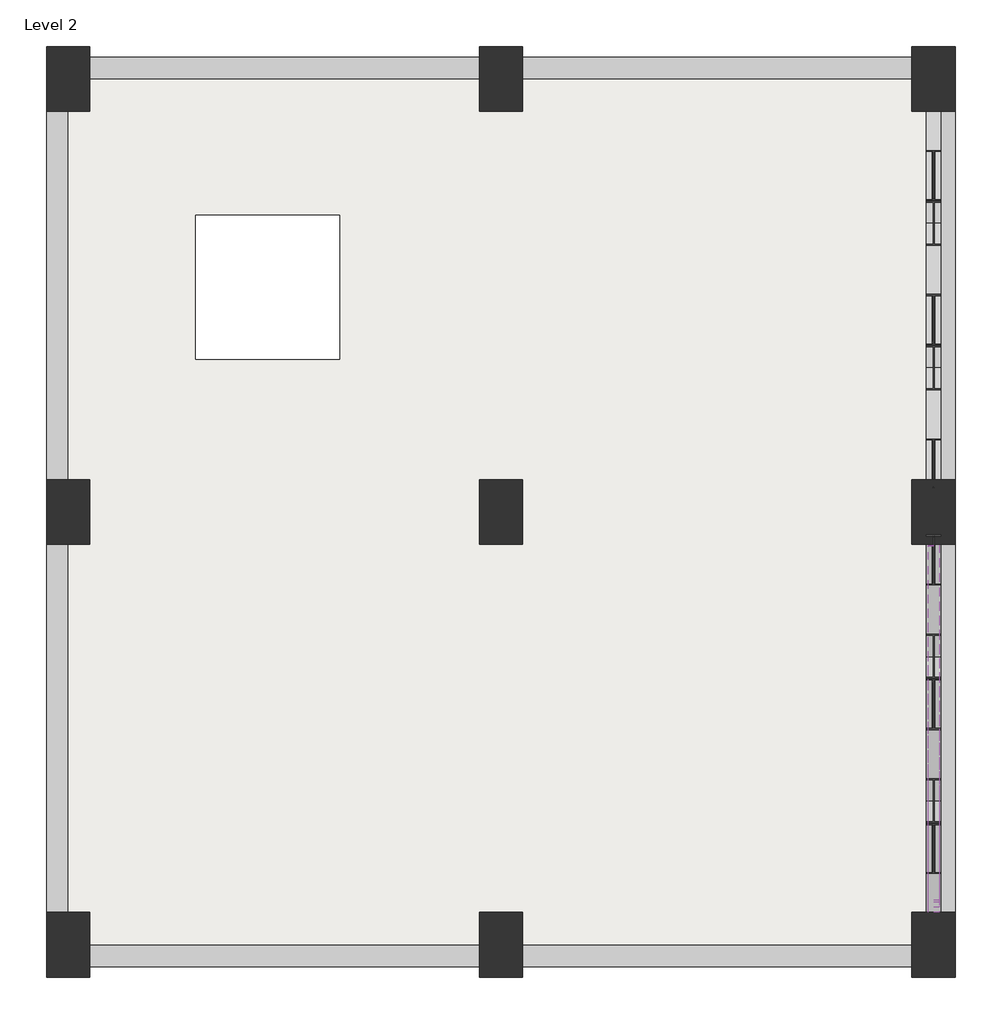
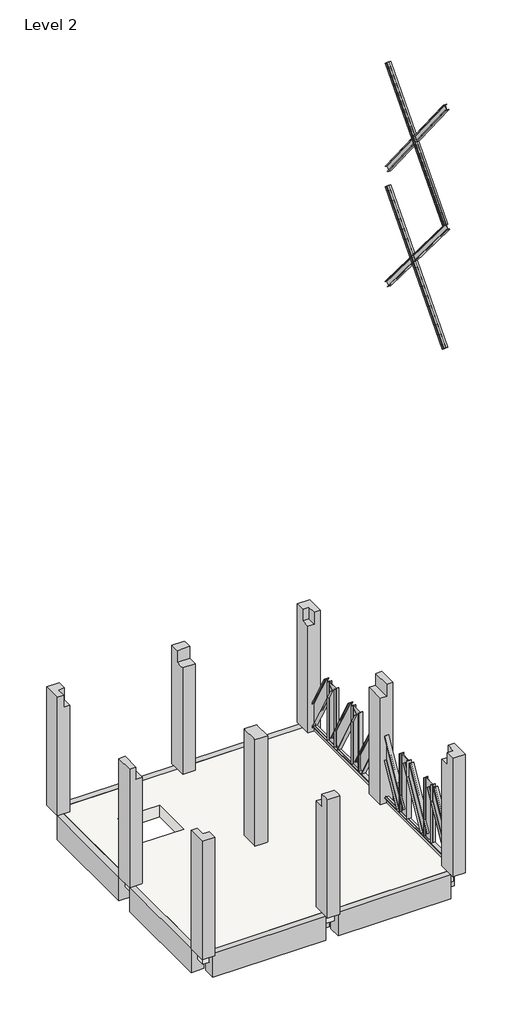
# One storey: 20 beams, 9 columns, 4 members, 1 slab.
"""IFC4 building model written with IfcOpenShell, lengths in millimetres."""

from ifc_helpers import new_model, si_unit, frame, origin, place, context, project, spatial, polyline, outline, extrude, faceted_brep, transform, mapped, element, save
from components import ub_universal_beams_ub305x102x25_07ba02ff, ub_universal_beams_ub305x102x25_e3bd1737, ub_universal_beams_ub305x102x25_1ef2d586, ub_universal_beams_ub305x102x25_1ce1eee3, ub_universal_beams_ub305x102x25_b0bcaaf9, ub_universal_beams_ub305x102x25_8854acc3, ub_universal_beams_ub127x76x13_debcaab1, ub_universal_beams_ub127x76x13_6b492b77, ub_universal_beams_ub127x76x13_5289bed7, ub_universal_beams_ub127x76x13_b97c8348

model = new_model("IFC4")

# Units and contexts
model_context = context("Model", 3, world=origin())
ifc_project = project(units=[si_unit("LENGTHUNIT", "METRE", prefix="MILLI")], contexts=[model_context])

# Site, building, storey
site = spatial("IfcSite", under=ifc_project)
building = spatial("IfcBuilding", under=site)
storey = spatial("IfcBuildingStorey", under=building, Name="Level 2", Elevation=3000.0)

# Beams
placement = place(None, origin())
element("IfcBeam", 1, ObjectType="Concrete-Rectangular Beam : 300 x 600mm", at=placement, inside=storey, context=model_context, shape_type="SweptSolid", body=[
    extrude(outline(polyline([(526.3372902, 2400.0), (226.3372902, 2400.0), (226.3372902, 2700.0), (376.3372902, 2700.0), (376.3372902, 3000.0), (526.3372902, 3000.0), (526.3372902, 2400.0)])), frame((2068.7595868, 0.0, 0.0), z_axis=(1.0, 0.0, 0.0), x_axis=(0.0, 1.0, 0.0)), (0.0, 0.0, 1.0), 2700.0),
    extrude(outline(polyline([(526.3372902, 2400.0), (226.3372902, 2400.0), (226.3372902, 2700.0), (376.3372902, 2700.0), (376.3372902, 3000.0), (526.3372902, 3000.0), (526.3372902, 2400.0)])), frame((-931.2404132, 0.0, 0.0), z_axis=(1.0, 0.0, 0.0), x_axis=(0.0, 1.0, 0.0)), (0.0, 0.0, 1.0), 2700.0),
])
element("IfcBeam", 2, ObjectType="Concrete-Rectangular Beam : 300 x 600mm", at=placement, inside=storey, context=model_context, shape_type="SweptSolid", body=[
    extrude(outline(polyline([(2400.0, 5068.7595868), (3000.0, 5068.7595868), (3000.0, 4918.7595868), (2700.0, 4918.7595868), (2700.0, 4768.7595868), (2400.0, 4768.7595868), (2400.0, 5068.7595868)])), frame((0.0, -2398.6627098, 0.0), z_axis=(0.0, 1.0, 0.0), x_axis=(0.0, 0.0, 1.0)), (0.0, 0.0, 1.0), 2550.0),
    extrude(outline(polyline([(2400.0, 5068.7595868), (3000.0, 5068.7595868), (3000.0, 4918.7595868), (2700.0, 4918.7595868), (2700.0, 4768.7595868), (2400.0, 4768.7595868), (2400.0, 5068.7595868)])), frame((0.0, -5398.6627098, 0.0), z_axis=(0.0, 1.0, 0.0), x_axis=(0.0, 0.0, 1.0)), (0.0, 0.0, 1.0), 2550.0),
])
element("IfcBeam", 3, ObjectType="Concrete-Rectangular Beam : 300 x 600mm", at=placement, inside=storey, context=model_context, shape_type="SweptSolid", body=[
    extrude(outline(polyline([(-5773.6627098, 2400.0), (-5773.6627098, 3000.0), (-5623.6627098, 3000.0), (-5623.6627098, 2700.0), (-5473.6627098, 2700.0), (-5473.6627098, 2400.0), (-5773.6627098, 2400.0)])), frame((2068.7595868, 0.0, 0.0), z_axis=(1.0, 0.0, 0.0), x_axis=(0.0, 1.0, 0.0)), (0.0, 0.0, 1.0), 2700.0),
    extrude(outline(polyline([(-5773.6627098, 2400.0), (-5773.6627098, 3000.0), (-5623.6627098, 3000.0), (-5623.6627098, 2700.0), (-5473.6627098, 2700.0), (-5473.6627098, 2400.0), (-5773.6627098, 2400.0)])), frame((-931.2404132, 0.0, 0.0), z_axis=(1.0, 0.0, 0.0), x_axis=(0.0, 1.0, 0.0)), (0.0, 0.0, 1.0), 2700.0),
])
element("IfcBeam", 4, ObjectType="Concrete-Rectangular Beam : 300 x 600mm", at=placement, inside=storey, context=model_context, shape_type="SweptSolid", body=[
    extrude(outline(polyline([(3000.0, -1231.2404132), (2400.0, -1231.2404132), (2400.0, -931.2404132), (2700.0, -931.2404132), (2700.0, -1081.2404132), (3000.0, -1081.2404132), (3000.0, -1231.2404132)])), frame((0.0, -5398.6627098, 0.0), z_axis=(0.0, 1.0, 0.0), x_axis=(0.0, 0.0, 1.0)), (0.0, 0.0, 1.0), 2550.0),
    extrude(outline(polyline([(3000.0, -1231.2404132), (2400.0, -1231.2404132), (2400.0, -931.2404132), (2700.0, -931.2404132), (2700.0, -1081.2404132), (3000.0, -1081.2404132), (3000.0, -1231.2404132)])), frame((0.0, -2398.6627098, 0.0), z_axis=(0.0, 1.0, 0.0), x_axis=(0.0, 0.0, 1.0)), (0.0, 0.0, 1.0), 2550.0),
])
element("IfcBeam", 5, ObjectType="Concrete-Rectangular Beam : 300 x 600mm", at=placement, inside=storey, context=model_context, shape_type="SweptSolid", body=[
    extrude(outline(polyline([(2068.7595868, -5398.6627098), (1768.7595868, -5398.6627098), (1768.7595868, -2848.6627098), (2068.7595868, -2848.6627098), (2068.7595868, -5398.6627098)])), frame((0.0, 0.0, 2400.0), z_axis=(0.0, 0.0, 1.0), x_axis=(1.0, 0.0, 0.0)), (0.0, 0.0, 1.0), 300.0),
    extrude(outline(polyline([(1768.7595868, 151.3372902), (2068.7595868, 151.3372902), (2068.7595868, -2398.6627098), (1768.7595868, -2398.6627098), (1768.7595868, 151.3372902)])), frame((0.0, 0.0, 2400.0), z_axis=(0.0, 0.0, 1.0), x_axis=(1.0, 0.0, 0.0)), (0.0, 0.0, 1.0), 300.0),
])
element("IfcBeam", 6, ObjectType="Concrete-Rectangular Beam : 300 x 600mm", at=placement, inside=storey, context=model_context, shape_type="SweptSolid", body=[
    extrude(outline(polyline([(4768.7595868, -2473.6627098), (4768.7595868, -2773.6627098), (2068.7595868, -2773.6627098), (2068.7595868, -2473.6627098), (4768.7595868, -2473.6627098)])), frame((0.0, 0.0, 2400.0), z_axis=(0.0, 0.0, 1.0), x_axis=(1.0, 0.0, 0.0)), (0.0, 0.0, 1.0), 300.0),
    extrude(outline(polyline([(-931.2404132, -2773.6627098), (-931.2404132, -2473.6627098), (1768.7595868, -2473.6627098), (1768.7595868, -2773.6627098), (-931.2404132, -2773.6627098)])), frame((0.0, 0.0, 2400.0), z_axis=(0.0, 0.0, 1.0), x_axis=(1.0, 0.0, 0.0)), (0.0, 0.0, 1.0), 300.0),
])
ub_universal_beams_ub305x102x25_shape = ub_universal_beams_ub305x102x25_07ba02ff(model_context)
element("IfcBeam", 7, ObjectType="UB-Universal Beams : UB305x102x25", at=placement, inside=storey, context=model_context, shape_type="MappedRepresentation", body=[
    mapped(ub_universal_beams_ub305x102x25_shape, transform((4918.7595868, -2623.6627098, 3000.0), x_axis=(0.0, 1.0, 0.0), y_axis=(-1.0, 0.0, 0.0), z_axis=(0.0, 0.0, 1.0))),
])
ub_universal_beams_ub305x102x25_2_shape = ub_universal_beams_ub305x102x25_e3bd1737(model_context)
element("IfcBeam", 8, ObjectType="UB-Universal Beams : UB305x102x25", at=placement, inside=storey, context=model_context, shape_type="MappedRepresentation", body=[
    mapped(ub_universal_beams_ub305x102x25_2_shape, transform((4918.7595868, -5623.6627098, 3900.0), x_axis=(0.0, 0.0, 1.0), y_axis=(1.0, 0.0, 0.0), z_axis=(0.0, 1.0, 0.0))),
])
element("IfcBeam", 9, ObjectType="UB-Universal Beams : UB305x102x25", at=placement, inside=storey, context=model_context, shape_type="MappedRepresentation", body=[
    mapped(ub_universal_beams_ub305x102x25_2_shape, transform((4918.7595868, -2623.6627098, 3900.0), x_axis=(0.0, 0.0, 1.0), y_axis=(1.0, 0.0, 0.0), z_axis=(0.0, 1.0, 0.0))),
])
element("IfcBeam", 10, ObjectType="UB-Universal Beams : UB305x102x25", at=placement, inside=storey, context=model_context, shape_type="MappedRepresentation", body=[
    mapped(ub_universal_beams_ub305x102x25_2_shape, transform((4918.7595868, 376.3372902, 3900.0), x_axis=(0.0, 0.0, 1.0), y_axis=(1.0, 0.0, 0.0), z_axis=(0.0, 1.0, 0.0))),
])
ub_universal_beams_ub305x102x25_3_shape = ub_universal_beams_ub305x102x25_1ef2d586(model_context)
element("IfcBeam", 11, ObjectType="UB-Universal Beams : UB305x102x25", at=placement, inside=storey, context=model_context, shape_type="MappedRepresentation", body=[
    mapped(ub_universal_beams_ub305x102x25_3_shape, transform((4918.7595868, -3623.6627098, 3900.0), x_axis=(0.0, 0.0, 1.0), y_axis=(1.0, 0.0, 0.0), z_axis=(0.0, 1.0, 0.0))),
])
element("IfcBeam", 12, ObjectType="UB-Universal Beams : UB305x102x25", at=placement, inside=storey, context=model_context, shape_type="MappedRepresentation", body=[
    mapped(ub_universal_beams_ub305x102x25_3_shape, transform((4918.7595868, -4623.6627098, 3900.0), x_axis=(0.0, 0.0, 1.0), y_axis=(1.0, 0.0, 0.0), z_axis=(0.0, 1.0, 0.0))),
])
element("IfcBeam", 13, ObjectType="UB-Universal Beams : UB305x102x25", at=placement, inside=storey, context=model_context, shape_type="MappedRepresentation", body=[
    mapped(ub_universal_beams_ub305x102x25_3_shape, transform((4918.7595868, -1623.6627098, 3900.0), x_axis=(0.0, 0.0, 1.0), y_axis=(1.0, 0.0, 0.0), z_axis=(0.0, 1.0, 0.0))),
])
element("IfcBeam", 14, ObjectType="UB-Universal Beams : UB305x102x25", at=placement, inside=storey, context=model_context, shape_type="MappedRepresentation", body=[
    mapped(ub_universal_beams_ub305x102x25_3_shape, transform((4918.7595868, -623.6627098, 3900.0), x_axis=(0.0, 0.0, 1.0), y_axis=(1.0, 0.0, 0.0), z_axis=(0.0, 1.0, 0.0))),
])
ub_universal_beams_ub305x102x25_4_shape = ub_universal_beams_ub305x102x25_1ce1eee3(model_context)
element("IfcBeam", 15, ObjectType="UB-Universal Beams : UB305x102x25", at=placement, inside=storey, context=model_context, shape_type="MappedRepresentation", body=[
    mapped(ub_universal_beams_ub305x102x25_4_shape, transform((4918.7595868, -3123.6627098, 3900.0), x_axis=(0.0, 0.4856429311786321, 0.8741572761215378), y_axis=(1.0, 0.0, 0.0), z_axis=(0.0, 0.8741572761215378, -0.4856429311786321))),
])
element("IfcBeam", 16, ObjectType="UB-Universal Beams : UB305x102x25", at=placement, inside=storey, context=model_context, shape_type="MappedRepresentation", body=[
    mapped(ub_universal_beams_ub305x102x25_4_shape, transform((4918.7595868, -123.6627098, 3900.0), x_axis=(0.0, 0.4856429311786321, -0.8741572761215378), y_axis=(1.0, 0.0, 0.0), z_axis=(0.0, -0.8741572761215378, -0.4856429311786321))),
])
ub_universal_beams_ub305x102x25_5_shape = ub_universal_beams_ub305x102x25_b0bcaaf9(model_context)
element("IfcBeam", 17, ObjectType="UB-Universal Beams : UB305x102x25", at=placement, inside=storey, context=model_context, shape_type="MappedRepresentation", body=[
    mapped(ub_universal_beams_ub305x102x25_5_shape, transform((4918.7595868, -5123.6627098, 3900.0), x_axis=(0.0, 0.4856429311786321, 0.8741572761215378), y_axis=(1.0, 0.0, 0.0), z_axis=(0.0, 0.8741572761215378, -0.4856429311786321))),
])
element("IfcBeam", 18, ObjectType="UB-Universal Beams : UB305x102x25", at=placement, inside=storey, context=model_context, shape_type="MappedRepresentation", body=[
    mapped(ub_universal_beams_ub305x102x25_5_shape, transform((4918.7595868, -2123.6627098, 3900.0), x_axis=(0.0, 0.4856429311786321, -0.8741572761215378), y_axis=(1.0, 0.0, 0.0), z_axis=(0.0, -0.8741572761215378, -0.4856429311786321))),
])
ub_universal_beams_ub305x102x25_6_shape = ub_universal_beams_ub305x102x25_8854acc3(model_context)
element("IfcBeam", 19, ObjectType="UB-Universal Beams : UB305x102x25", at=placement, inside=storey, context=model_context, shape_type="MappedRepresentation", body=[
    mapped(ub_universal_beams_ub305x102x25_6_shape, transform((4918.7595868, -4123.6627098, 3900.0), x_axis=(0.0, 0.4856429311786321, 0.8741572761215378), y_axis=(1.0, 0.0, 0.0), z_axis=(0.0, 0.8741572761215378, -0.4856429311786321))),
])
element("IfcBeam", 20, ObjectType="UB-Universal Beams : UB305x102x25", at=placement, inside=storey, context=model_context, shape_type="MappedRepresentation", body=[
    mapped(ub_universal_beams_ub305x102x25_6_shape, transform((4918.7595868, -1123.6627098, 3900.0), x_axis=(0.0, 0.4856429311786321, -0.8741572761215378), y_axis=(1.0, 0.0, 0.0), z_axis=(0.0, -0.8741572761215378, -0.4856429311786321))),
])

# Columns
element("IfcColumn", 21, ObjectType="Concrete-Rectangular-Column : 300 x 450mm", at=placement, inside=storey, context=model_context, shape_type="Brep", body=[
    faceted_brep([(-1231.2404132, -5848.6627098, 6000.0), (-931.2404132, -5848.6627098, 6000.0), (-931.2404132, -5623.6627098, 6000.0), (-1081.2404132, -5623.6627098, 6000.0), (-1081.2404132, -5398.6627098, 6000.0), (-1231.2404132, -5398.6627098, 6000.0), (-1231.2404132, -5848.6627098, 3000.0), (-1231.2404132, -5398.6627098, 3000.0), (-931.2404132, -5398.6627098, 3000.0), (-931.2404132, -5848.6627098, 3000.0), (-931.2404132, -5398.6627098, 5700.0), (-931.2404132, -5623.6627098, 5700.0), (-1081.2404132, -5398.6627098, 5700.0), (-1081.2404132, -5623.6627098, 5700.0)], [[[0, 1, 2, 3, 4, 5]], [[6, 7, 8, 9]], [[1, 0, 6, 9]], [[9, 8, 10, 11, 2, 1]], [[8, 7, 5, 4, 12, 10]], [[0, 5, 7, 6]], [[12, 13, 11, 10]], [[13, 3, 2, 11]], [[3, 13, 12, 4]]]),
])
element("IfcColumn", 22, ObjectType="Concrete-Rectangular-Column : 300 x 450mm", at=placement, inside=storey, context=model_context, shape_type="Brep", body=[
    faceted_brep([(1768.7595868, -5848.6627098, 6000.0), (2068.7595868, -5848.6627098, 6000.0), (2068.7595868, -5773.6627098, 6000.0), (2068.7595868, -5623.6627098, 6000.0), (1768.7595868, -5623.6627098, 6000.0), (1768.7595868, -5773.6627098, 6000.0), (1768.7595868, -5848.6627098, 3000.0), (1768.7595868, -5398.6627098, 3000.0), (2068.7595868, -5398.6627098, 3000.0), (2068.7595868, -5848.6627098, 3000.0), (2068.7595868, -5398.6627098, 5700.0), (2068.7595868, -5473.6627098, 5700.0), (2068.7595868, -5623.6627098, 5700.0), (1768.7595868, -5398.6627098, 5700.0), (1768.7595868, -5623.6627098, 5700.0), (1768.7595868, -5473.6627098, 5700.0)], [[[0, 1, 2, 3, 4, 5]], [[6, 7, 8, 9]], [[1, 0, 6, 9]], [[9, 8, 10, 11, 12, 3, 2, 1]], [[8, 7, 13, 10]], [[7, 6, 0, 5, 4, 14, 15, 13]], [[14, 12, 11, 10, 13, 15]], [[12, 14, 4, 3]]]),
])
element("IfcColumn", 23, ObjectType="Concrete-Rectangular-Column : 300 x 450mm", at=placement, inside=storey, context=model_context, shape_type="Brep", body=[
    faceted_brep([(4768.7595868, -5848.6627098, 6000.0), (5068.7595868, -5848.6627098, 6000.0), (5068.7595868, -5398.6627098, 6000.0), (4918.7595868, -5398.6627098, 6000.0), (4918.7595868, -5623.6627098, 6000.0), (4768.7595868, -5623.6627098, 6000.0), (4768.7595868, -5848.6627098, 3000.0), (4768.7595868, -5398.6627098, 3000.0), (5068.7595868, -5398.6627098, 3000.0), (5068.7595868, -5848.6627098, 3000.0), (4768.7595868, -5398.6627098, 5700.0), (4918.7595868, -5398.6627098, 5700.0), (4768.7595868, -5623.6627098, 5700.0), (4918.7595868, -5623.6627098, 5700.0)], [[[0, 1, 2, 3, 4, 5]], [[6, 7, 8, 9]], [[1, 0, 6, 9]], [[2, 1, 9, 8]], [[8, 7, 10, 11, 3, 2]], [[7, 6, 0, 5, 12, 10]], [[12, 13, 11, 10]], [[13, 4, 3, 11]], [[4, 13, 12, 5]]]),
])
element("IfcColumn", 24, ObjectType="Concrete-Rectangular-Column : 300 x 450mm", at=placement, inside=storey, context=model_context, shape_type="Brep", body=[
    faceted_brep([(-1231.2404132, -2398.6627098, 6000.0), (-1231.2404132, -2848.6627098, 6000.0), (-1081.2404132, -2848.6627098, 6000.0), (-1081.2404132, -2398.6627098, 6000.0), (-1231.2404132, -2848.6627098, 3000.0), (-1231.2404132, -2398.6627098, 3000.0), (-931.2404132, -2398.6627098, 3000.0), (-931.2404132, -2848.6627098, 3000.0), (-931.2404132, -2848.6627098, 5400.0), (-931.2404132, -2848.6627098, 5700.0), (-1081.2404132, -2848.6627098, 5700.0), (-1231.2404132, -2848.6627098, 5400.0), (-931.2404132, -2398.6627098, 5400.0), (-931.2404132, -2398.6627098, 5700.0), (-1231.2404132, -2398.6627098, 5400.0), (-1081.2404132, -2398.6627098, 5700.0)], [[[0, 1, 2, 3]], [[4, 5, 6, 7]], [[4, 7, 8, 9, 10, 2, 1, 11]], [[7, 6, 12, 13, 9, 8]], [[6, 5, 14, 0, 3, 15, 13, 12]], [[1, 0, 14, 5, 4, 11]], [[15, 10, 9, 13]], [[10, 15, 3, 2]]]),
])
element("IfcColumn", 25, ObjectType="Concrete-Rectangular-Column : 300 x 450mm", at=placement, inside=storey, context=model_context, shape_type="Brep", body=[
    faceted_brep([(1768.7595868, -2848.6627098, 3000.0), (1768.7595868, -2398.6627098, 3000.0), (2068.7595868, -2398.6627098, 3000.0), (2068.7595868, -2848.6627098, 3000.0), (2068.7595868, -2848.6627098, 5400.0), (2068.7595868, -2848.6627098, 5700.0), (1768.7595868, -2848.6627098, 5700.0), (1768.7595868, -2848.6627098, 5400.0), (2068.7595868, -2398.6627098, 5400.0), (2068.7595868, -2398.6627098, 5700.0), (2068.7595868, -2473.6627098, 5700.0), (2068.7595868, -2773.6627098, 5700.0), (1768.7595868, -2398.6627098, 5400.0), (1768.7595868, -2398.6627098, 5700.0), (1768.7595868, -2773.6627098, 5700.0), (1768.7595868, -2473.6627098, 5700.0)], [[[0, 1, 2, 3]], [[0, 3, 4, 5, 6, 7]], [[3, 2, 8, 9, 10, 11, 5, 4]], [[2, 1, 12, 13, 9, 8]], [[1, 0, 7, 6, 14, 15, 13, 12]], [[6, 5, 11, 10, 9, 13, 15, 14]]]),
])
element("IfcColumn", 26, ObjectType="Concrete-Rectangular-Column : 300 x 450mm", at=placement, inside=storey, context=model_context, shape_type="Brep", body=[
    faceted_brep([(5068.7595868, -2848.6627098, 6000.0), (5068.7595868, -2398.6627098, 6000.0), (4918.7595868, -2398.6627098, 6000.0), (4918.7595868, -2848.6627098, 6000.0), (4768.7595868, -2848.6627098, 3000.0), (4768.7595868, -2398.6627098, 3000.0), (5068.7595868, -2398.6627098, 3000.0), (5068.7595868, -2848.6627098, 3000.0), (5068.7595868, -2848.6627098, 5400.0), (4918.7595868, -2848.6627098, 5700.0), (4768.7595868, -2848.6627098, 5700.0), (4768.7595868, -2848.6627098, 5400.0), (5068.7595868, -2398.6627098, 5400.0), (4768.7595868, -2398.6627098, 5400.0), (4768.7595868, -2398.6627098, 5700.0), (4918.7595868, -2398.6627098, 5700.0)], [[[0, 1, 2, 3]], [[4, 5, 6, 7]], [[4, 7, 8, 0, 3, 9, 10, 11]], [[1, 0, 8, 7, 6, 12]], [[6, 5, 13, 14, 15, 2, 1, 12]], [[5, 4, 11, 10, 14, 13]], [[9, 15, 14, 10]], [[15, 9, 3, 2]]]),
])
element("IfcColumn", 27, ObjectType="Concrete-Rectangular-Column : 300 x 450mm", at=placement, inside=storey, context=model_context, shape_type="Brep", body=[
    faceted_brep([(-931.2404132, 601.3372902, 6000.0), (-1231.2404132, 601.3372902, 6000.0), (-1231.2404132, 151.3372902, 6000.0), (-1081.2404132, 151.3372902, 6000.0), (-1081.2404132, 376.3372902, 6000.0), (-931.2404132, 376.3372902, 6000.0), (-1231.2404132, 151.3372902, 3000.0), (-1231.2404132, 601.3372902, 3000.0), (-931.2404132, 601.3372902, 3000.0), (-931.2404132, 151.3372902, 3000.0), (-931.2404132, 151.3372902, 5700.0), (-1081.2404132, 151.3372902, 5700.0), (-931.2404132, 376.3372902, 5700.0), (-1081.2404132, 376.3372902, 5700.0)], [[[0, 1, 2, 3, 4, 5]], [[6, 7, 8, 9]], [[6, 9, 10, 11, 3, 2]], [[9, 8, 0, 5, 12, 10]], [[1, 0, 8, 7]], [[2, 1, 7, 6]], [[12, 13, 11, 10]], [[13, 4, 3, 11]], [[4, 13, 12, 5]]]),
])
element("IfcColumn", 28, ObjectType="Concrete-Rectangular-Column : 300 x 450mm", at=placement, inside=storey, context=model_context, shape_type="Brep", body=[
    faceted_brep([(2068.7595868, 601.3372902, 6000.0), (1768.7595868, 601.3372902, 6000.0), (1768.7595868, 526.3372902, 6000.0), (1768.7595868, 376.3372902, 6000.0), (2068.7595868, 376.3372902, 6000.0), (2068.7595868, 526.3372902, 6000.0), (1768.7595868, 151.3372902, 3000.0), (1768.7595868, 601.3372902, 3000.0), (2068.7595868, 601.3372902, 3000.0), (2068.7595868, 151.3372902, 3000.0), (2068.7595868, 151.3372902, 5700.0), (1768.7595868, 151.3372902, 5700.0), (2068.7595868, 376.3372902, 5700.0), (2068.7595868, 226.3372902, 5700.0), (1768.7595868, 226.3372902, 5700.0), (1768.7595868, 376.3372902, 5700.0)], [[[0, 1, 2, 3, 4, 5]], [[6, 7, 8, 9]], [[6, 9, 10, 11]], [[9, 8, 0, 5, 4, 12, 13, 10]], [[1, 0, 8, 7]], [[7, 6, 11, 14, 15, 3, 2, 1]], [[12, 15, 14, 11, 10, 13]], [[15, 12, 4, 3]]]),
])
element("IfcColumn", 29, ObjectType="Concrete-Rectangular-Column : 300 x 450mm", at=placement, inside=storey, context=model_context, shape_type="Brep", body=[
    faceted_brep([(5068.7595868, 151.3372902, 6000.0), (5068.7595868, 601.3372902, 6000.0), (4768.7595868, 601.3372902, 6000.0), (4768.7595868, 376.3372902, 6000.0), (4918.7595868, 376.3372902, 6000.0), (4918.7595868, 151.3372902, 6000.0), (4768.7595868, 151.3372902, 3000.0), (4768.7595868, 601.3372902, 3000.0), (5068.7595868, 601.3372902, 3000.0), (5068.7595868, 151.3372902, 3000.0), (4918.7595868, 151.3372902, 5700.0), (4768.7595868, 151.3372902, 5700.0), (4768.7595868, 376.3372902, 5700.0), (4918.7595868, 376.3372902, 5700.0)], [[[0, 1, 2, 3, 4, 5]], [[6, 7, 8, 9]], [[6, 9, 0, 5, 10, 11]], [[1, 0, 9, 8]], [[2, 1, 8, 7]], [[7, 6, 11, 12, 3, 2]], [[13, 12, 11, 10]], [[4, 13, 10, 5]], [[13, 4, 3, 12]]]),
])

# Members
ub_universal_beams_ub127x76x13_shape = ub_universal_beams_ub127x76x13_debcaab1(model_context)
element("IfcMember", 30, ObjectType="UB-Universal Beams : UB127x76x13", at=placement, inside=storey, context=model_context, shape_type="MappedRepresentation", body=[
    mapped(ub_universal_beams_ub127x76x13_shape, transform((4918.7595868, -4111.8389624, 20600.0), x_axis=(0.0, -0.6255639528367075, 0.7801728916793468), y_axis=(1.0, 0.0, 0.0), z_axis=(0.0, 0.7801728916793468, 0.6255639528367075))),
])
ub_universal_beams_ub127x76x13_2_shape = ub_universal_beams_ub127x76x13_6b492b77(model_context)
element("IfcMember", 31, ObjectType="UB-Universal Beams : UB127x76x13", at=placement, inside=storey, context=model_context, shape_type="MappedRepresentation", body=[
    mapped(ub_universal_beams_ub127x76x13_2_shape, transform((4918.7595868, -3953.42931, 20600.0), x_axis=(0.0, 0.6633692943777195, 0.7482921750738855), y_axis=(-1.0, 0.0, 0.0), z_axis=(0.0, -0.7482921750738855, 0.6633692943777195))),
])
ub_universal_beams_ub127x76x13_3_shape = ub_universal_beams_ub127x76x13_5289bed7(model_context)
element("IfcMember", 32, ObjectType="UB-Universal Beams : UB127x76x13", at=placement, inside=storey, context=model_context, shape_type="MappedRepresentation", body=[
    mapped(ub_universal_beams_ub127x76x13_3_shape, transform((4918.7595868, -3987.3365723, 17470.50801), x_axis=(0.0, 0.6417839133356917, -0.7668855250841063), y_axis=(-1.0, 0.0, 0.0), z_axis=(0.0, 0.7668855250841063, 0.6417839133356917))),
])
ub_universal_beams_ub127x76x13_4_shape = ub_universal_beams_ub127x76x13_b97c8348(model_context)
element("IfcMember", 33, ObjectType="UB-Universal Beams : UB127x76x13", at=placement, inside=storey, context=model_context, shape_type="MappedRepresentation", body=[
    mapped(ub_universal_beams_ub127x76x13_4_shape, transform((4918.7595868, -3946.516498, 17476.6450694), x_axis=(0.0, -0.6614316775001309, -0.7500054239799623), y_axis=(1.0, 0.0, 0.0), z_axis=(0.0, -0.7500054239799623, 0.6614316775001309))),
])

# Slab
element("IfcSlab", 34, ObjectType="Generic 300mm", at=placement, inside=storey, context=model_context, shape_type="Brep", body=[
    faceted_brep([(4918.7595868, 376.3372902, 2700.0), (4918.7595868, 151.3372902, 2700.0), (4918.7595868, -2398.6627098, 2700.0), (4918.7595868, -2848.6627098, 2700.0), (4918.7595868, -5398.6627098, 2700.0), (4918.7595868, -5623.6627098, 2700.0), (4768.7595868, -5623.6627098, 2700.0), (2068.7595868, -5623.6627098, 2700.0), (1768.7595868, -5623.6627098, 2700.0), (-931.2404132, -5623.6627098, 2700.0), (-1081.2404132, -5623.6627098, 2700.0), (-1081.2404132, -5398.6627098, 2700.0), (-1081.2404132, -2848.6627098, 2700.0), (-1081.2404132, -2398.6627098, 2700.0), (-1081.2404132, 151.3372902, 2700.0), (-1081.2404132, 376.3372902, 2700.0), (-931.2404132, 376.3372902, 2700.0), (1768.7595868, 376.3372902, 2700.0), (2068.7595868, 376.3372902, 2700.0), (4768.7595868, 376.3372902, 2700.0), (-198.5229478, -1566.5574371, 2700.0), (801.4770522, -1566.5574371, 2700.0), (801.4770522, -566.5574371, 2700.0), (-198.5229478, -566.5574371, 2700.0), (4918.7595868, -5623.6627098, 3000.0), (4918.7595868, -5398.6627098, 3000.0), (4918.7595868, -2848.6627098, 3000.0), (4918.7595868, -2398.6627098, 3000.0), (4918.7595868, 151.3372902, 3000.0), (4918.7595868, 376.3372902, 3000.0), (4768.7595868, 376.3372902, 3000.0), (2068.7595868, 376.3372902, 3000.0), (1768.7595868, 376.3372902, 3000.0), (-931.2404132, 376.3372902, 3000.0), (-1081.2404132, 376.3372902, 3000.0), (-1081.2404132, 151.3372902, 3000.0), (-1081.2404132, -2398.6627098, 3000.0), (-1081.2404132, -2848.6627098, 3000.0), (-1081.2404132, -5398.6627098, 3000.0), (-1081.2404132, -5623.6627098, 3000.0), (-931.2404132, -5623.6627098, 3000.0), (1768.7595868, -5623.6627098, 3000.0), (2068.7595868, -5623.6627098, 3000.0), (4768.7595868, -5623.6627098, 3000.0), (801.4770522, -1566.5574371, 3000.0), (-198.5229478, -1566.5574371, 3000.0), (-198.5229478, -566.5574371, 3000.0), (801.4770522, -566.5574371, 3000.0)], [[[0, 1, 2, 3, 4, 5, 6, 7, 8, 9, 10, 11, 12, 13, 14, 15, 16, 17, 18, 19], [20, 21, 22, 23]], [[24, 25, 26, 27, 28, 29, 30, 31, 32, 33, 34, 35, 36, 37, 38, 39, 40, 41, 42, 43], [44, 45, 46, 47]], [[5, 4, 3, 2, 1, 0, 29, 28, 27, 26, 25, 24]], [[10, 9, 8, 7, 6, 5, 24, 43, 42, 41, 40, 39]], [[15, 14, 13, 12, 11, 10, 39, 38, 37, 36, 35, 34]], [[0, 19, 18, 17, 16, 15, 34, 33, 32, 31, 30, 29]], [[20, 45, 44, 21]], [[21, 44, 47, 22]], [[22, 47, 46, 23]], [[45, 20, 23, 46]]]),
])

save(model, "model.ifc")

# Revit data of these elements
# Type "Concrete-Rectangular Beam : 300 x 600mm"
#   Length [instance default] = 1.524 m
#   b = 0.3 m
#   h = 0.6 m
#   Structural Material [instance default] = Concrete, Cast-in-Place gray
#   Assembly Code = ""
# Type "UB-Universal Beams : UB305x102x25"
#   Section Name Key = "UB305X102X25"
#   Width = 10.16 cm
#   Web Thickness = 0.58 cm
#   Web Fillet = 0.76 cm
#   Warping Constant = 27300.0 cm⁶
#   Torsional Moment of Inertia = 4.77 cm⁴
#   Section Area = 31.6 cm²
#   Plastic Modulus weak axis = 39.0 cm³
#   Plastic Modulus strong axis = 342.0 cm³
#   Nominal Weight = 24.7999 kgf/m
#   Moment of Inertia weak axis = 123.00 cm⁴
#   Moment of Inertia strong axis = 4455.00 cm⁴
#   Height = 30.51 cm
#   Flange Thickness = 0.7 cm
#   Elastic Modulus weak axis = 24.2 cm³
#   Elastic Modulus strong axis = 292.0 cm³
#   Centroid Vertical = 15.255 cm
#   Centroid Horizontal = 5.08 cm
#   Bolt Spacing = 5.4 cm
#   Length [instance default] = 1.5 m
#   Structural Material [instance default] = Metal - Steel 43-275
#   Type Comments = ""
#   Assembly Code = ""
# Type "Concrete-Rectangular-Column : 300 x 450mm"
#   b = 0.3 m
#   h = 0.45 m
#   Structural Material [instance default] = Concrete, Cast-in-Place gray
# Type "UB-Universal Beams : UB127x76x13"
#   Section Name Key = "UB127X76X13"
#   Width = 7.6 cm
#   Web Thickness = 0.4 cm
#   Web Fillet = 0.76 cm
#   Warping Constant = 2000.0 cm⁶
#   Torsional Moment of Inertia = 2.85 cm⁴
#   Section Area = 16.5 cm²
#   Plastic Modulus weak axis = 22.6 cm³
#   Plastic Modulus strong axis = 84.2 cm³
#   Nominal Weight = 13.00 kgf/m
#   Moment of Inertia weak axis = 55.70 cm⁴
#   Moment of Inertia strong axis = 473.00 cm⁴
#   Height = 12.7 cm
#   Flange Thickness = 0.76 cm
#   Elastic Modulus weak axis = 14.7 cm³
#   Elastic Modulus strong axis = 74.6 cm³
#   Centroid Vertical = 6.35 cm
#   Centroid Horizontal = 3.8 cm
#   Bolt Spacing = 4.0 cm
#   Length [instance default] = 1.5 m
#   Structural Material [instance default] = Metal - Steel 43-275
#   Type Comments = ""
#   Assembly Code = ""
# Type "Generic 300mm"
#   Function = 0
#   Layers, outside or top first: 0.3 m no material (function 1)
# Elements 1, 2, 3, 4, 5, 6 (IfcBeam, "Concrete-Rectangular Beam : 300 x 600mm")
#   Structural Material = Concrete, Cast-in-Place gray
#   Phase Created = New Construction
#   Materials on its faces: "Concrete, Cast-in-Place gray"
# Elements 7, 8, 9, 10, 11, 12, 13, 14, 15, 16, 17, 18, 19, 20 (IfcBeam, "UB-Universal Beams : UB305x102x25")
#   Structural Material = Metal - Steel 43-275
#   Phase Created = New Construction
#   Materials on its faces: "Metal - Steel 43-275"
# Elements 21, 22, 23, 24, 25, 26, 27, 28, 29 (IfcColumn, "Concrete-Rectangular-Column : 300 x 450mm")
#   Structural Material = Concrete, Cast-in-Place gray
#   Phase Created = New Construction
#   Materials on its faces: "Concrete, Cast-in-Place gray"
# Elements 30, 31, 32, 33 (IfcMember, "UB-Universal Beams : UB127x76x13")
#   Structural Material = Metal - Steel 43-275
#   Phase Created = New Construction
#   Materials on its faces: "Metal - Steel 43-275"
# Element 34 (IfcSlab, "Generic 300mm")
#   Height Offset From Level = 0 m
#   built-in parameter 1001954 = 1
#   Phase Created = New Construction
#   Materials on its faces: "Default Floor"
# Materials
#   "Concrete, Cast-in-Place gray": class "Concrete", colour RGB 192 192 192, transparency 0, Description = "Cast-in-place concrete", Cost = 0
#   "Metal - Steel 43-275": class "Metal", colour RGB 247 247 247, transparency 0, Cost = 0
#   "Default Floor": colour RGB 127 127 127, transparency 0, Cost = 0
